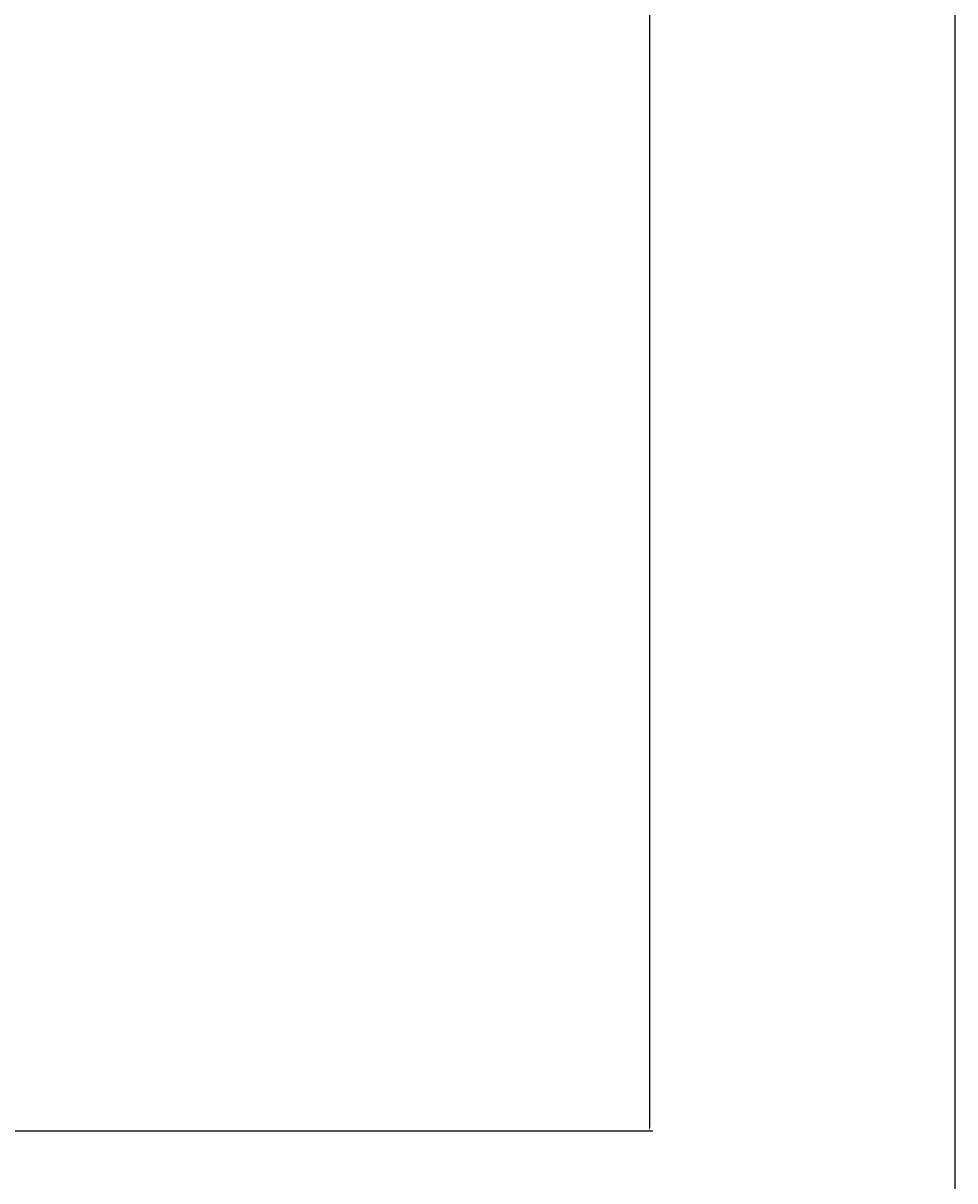
# Model space of a CAD drawing. Units: inches. Extents: x 1601 to 2297, y 1496 to 2631.
# Tile 20 of 57: x 2242 to 2297, y 1632 to 1701. Entities that reach past the tile are written whole.
import ezdxf

# ---------------------------------------------------------------- set-up
doc = ezdxf.new("R2010")
doc.units = ezdxf.units.IN
doc.layers.add('A-ANNO-DIMS', color=2, linetype='Continuous', lineweight=18)
doc.layers.add('A-ANNO-TTLB', color=7, linetype='Continuous', lineweight=25)
doc.styles.get("Standard").update_dxf_attribs({"font": 'arial.ttf'})
doc.dimstyles.get("Standard").update_dxf_attribs({"dimtxt": 0.18, "dimasz": 0.18, "dimexe": 0.18, "dimexo": 0.0625, "dimgap": 0.09, "dimtad": 0, "dimtih": 1, "dimtoh": 1, "dimdec": 4, "dimzin": 0, "dimdsep": 46, "dimtxsty": 'Standard', "dimcen": 0.09, "dimadec": 0, "dimazin": 0, "dimtfac": 1, "dimtdec": 4, "dimtofl": 0, "dimtmove": 0, "dimatfit": 3, "dimfxl": 1, "dimtolj": 1, "dimtzin": 0, "dimarcsym": 0})

# ---------------------------------------------------------------- blocks, each defined once
blk = doc.blocks.new('*D29')
at = {"layer": 'A-ANNO-DIMS', "color": 0, "lineweight": -2, "transparency": 16777216}
for p, q in [((2230.6, 2532.325), (2279.267, 2532.325)), ((2279.087, 2532.145), (2279.087, 2084.007)), ((2279.087, 1635.505), (2279.087, 2083.643)), ((2230.6, 1635.325), (2279.267, 1635.325))]:
    blk.add_line(p, q, dxfattribs=at)
at = {"layer": 'A-ANNO-DIMS', "color": 0, "transparency": 16777216}
for points in [[(2279.057, 2532.145), (2279.117, 2532.145), (2279.087, 2532.325)], [(2279.057, 1635.505), (2279.117, 1635.505), (2279.087, 1635.325)]]:
    blk.add_solid(points, dxfattribs=at)
at = {"layer": 'Defpoints', "color": 0, "transparency": 16777216}
for p in [(2230.537, 2532.325), (2279.087, 2532.325), (2230.537, 1635.325)]:
    blk.add_point(p, dxfattribs=at)
at = {"layer": 'A-ANNO-DIMS', "color": 0, "transparency": 16777216, "insert": (2279.087, 2083.825), "char_height": 0.18, "attachment_point": 5}
blk.add_mtext('\\A1;897', dxfattribs=at)

msp = doc.modelspace()

# ---------------------------------------------------------------- linework, layer by layer
at = {"layer": 'A-ANNO-TTLB'}
msp.add_lwpolyline([(1600.5933, 2631.1477), (2297.129, 2631.1477), (2297.129, 1496.1026), (1600.5933, 1496.1026)], close=True, dxfattribs=at)

# ---------------------------------------------------------------- dimensions: what is measured, and where the dimension line sits
at = {"layer": 'A-ANNO-DIMS'}
dim = msp.add_linear_dim(base=(2279.0873, 2532.3254), p1=(2230.5373, 1635.3254), p2=(2230.5373, 2532.3254), angle=90, dimstyle='Standard', override={"dimdec": 0, "dimlfac": 1, "dimrnd": 0, "dimzin": 0, "dimdsep": 46, "dimlunit": 2}, dxfattribs=at)
dim.commit()
dim.dimension.update_dxf_attribs({"geometry": '*D29', "text_midpoint": (2279.0873, 2083.8254)})

doc.saveas('drawing.dxf')
